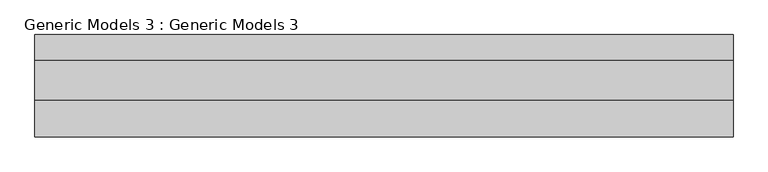
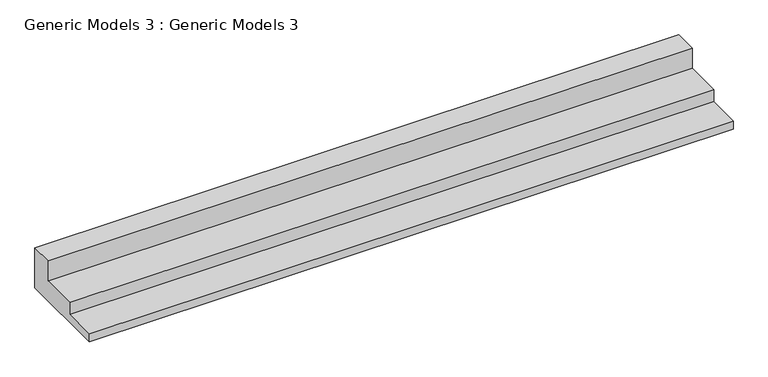
"""IFC4 building model written with IfcOpenShell, lengths in millimetres: proxy geometry, Generic Models 3 : Generic Models 3."""

from ifc_helpers import new_model, si_unit, frame, origin, place, context, project, spatial, polyline, outline, extrude, source, transform, mapped, element, save


def generic_models_3_generic_models_3_935cad4b(model_context):
    return source(origin(), model_context, "Body", "SweptSolid", [
        extrude(outline(polyline([(-7265.2302427, 0.0), (-7830.3802427, 0.0), (-7830.3802427, 50.8), (-7627.1802427, 50.8), (-7627.1802427, 127.0), (-7404.9302427, 127.0), (-7404.9302427, 254.0), (-7265.2302427, 254.0), (-7265.2302427, 0.0)])), frame((-4872.2564261, 0.0, 0.0), z_axis=(1.0, 0.0, 0.0), x_axis=(0.0, 1.0, 0.0)), (0.0, 0.0, 1.0), 3859.789196),
    ])


if __name__ == "__main__":
    model = new_model("IFC4")
    model_context = context("Model", 3, world=origin())
    ifc_project = project(units=[si_unit("LENGTHUNIT", "METRE", prefix="MILLI")], contexts=[model_context])
    site = spatial("IfcSite", under=ifc_project)
    building = spatial("IfcBuilding", under=site)
    placement = place(None, origin())
    generic_models_3_generic_models_3_shape = generic_models_3_generic_models_3_935cad4b(model_context)
    element("IfcBuildingElementProxy", 1, Name="Generic Models 3 : Generic Models 3", ObjectType="Generic Models 3 : Generic Models 3", at=placement, inside=building, context=model_context, shape_type="MappedRepresentation", body=[
        mapped(generic_models_3_generic_models_3_shape, transform((0.0, 0.0, 0.0), x_axis=(1.0, 0.0, 0.0), y_axis=(0.0, 1.0, 0.0), z_axis=(0.0, 0.0, 1.0))),
    ])
    save(model, "model.ifc")

# Revit data of these elements
# Element 1 (IfcBuildingElementProxy, "Generic Models 3 : Generic Models 3")
#   Materials on its faces: "Laminate, Ivory, Matte"
# Materials
#   "Laminate, Ivory, Matte": class "Plastic", colour RGB 247 247 239, transparency 0, Description = "Plastic Laminate - Ivory, Matte", Cost = 0
